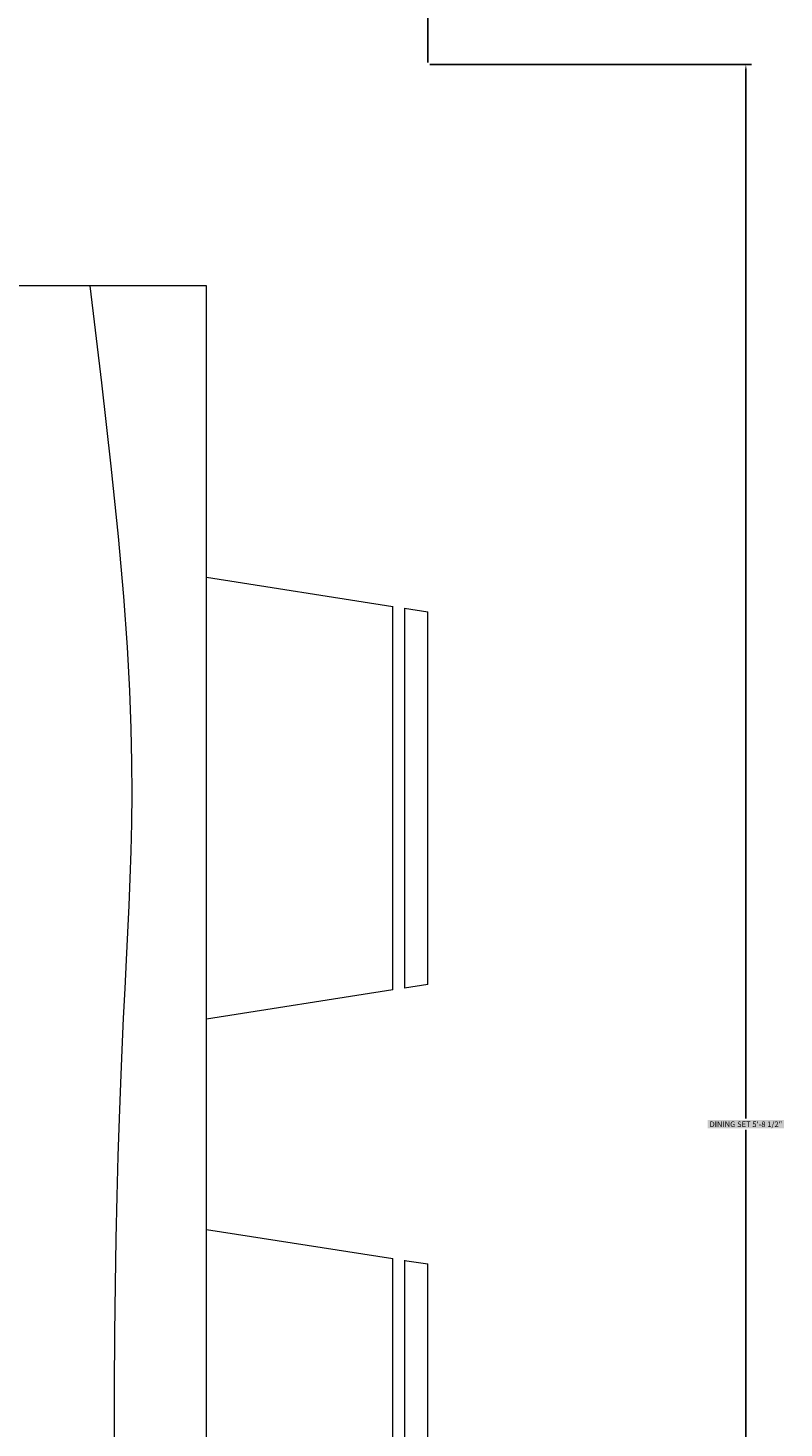
# Model space of a CAD drawing. Units: inches. Extents: x -301 to 715, y -607 to 364.
# Tile 112 of 141: x -12 to 12, y 147 to 192. Entities that reach past the tile are written whole.
import ezdxf

# ---------------------------------------------------------------- set-up
doc = ezdxf.new("R2010")
doc.units = ezdxf.units.IN
doc.header["$MEASUREMENT"] = 0
doc.layers.add('A-ANNO-DIMS', color=2, linetype='Continuous', lineweight=18)
doc.layers.add('A-FURN', color=8, linetype='Continuous', lineweight=18)
doc.styles.get("Standard").update_dxf_attribs({"font": 'arial.ttf'})
doc.dimstyles.get("Standard").update_dxf_attribs({"dimtxt": 0.18, "dimasz": 0.18, "dimexe": 0.18, "dimexo": 0.0625, "dimgap": 0.09, "dimtad": 0, "dimtih": 1, "dimtoh": 1, "dimdec": 1, "dimzin": 0, "dimdsep": 46, "dimlunit": 4, "dimtxsty": 'Standard', "dimcen": 0.09, "dimclrd": 3, "dimclre": 4, "dimclrt": 6, "dimadec": 0, "dimazin": 0, "dimtfac": 1, "dimtdec": 1, "dimtofl": 0, "dimtmove": 0, "dimatfit": 3, "dimfxl": 1, "dimtfill": 2, "dimtfillclr": 51, "dimtolj": 1, "dimtzin": 0, "dimarcsym": 0})

# ---------------------------------------------------------------- blocks, each defined once
blk = doc.blocks.new('Dining Set - 36 x 72 in.')
for p, q in [((36, -18), (36, 18)), ((-36, -18), (36, -18)), ((-4.5152, -17.99762), (-5.7655, -25.99928)), ((5.7657, -26.0006), (4.5153, -17.99762)), ((23.4848, -17.99762), (22.2345, -25.99928)), ((-22.2304, -26), (-5.7608, -26)), ((5.7696, -26), (22.2392, -26)), ((-5.8416, -26.5), (-22.1534, -26.5)), ((-5.8437, -26.49967), (-6, -27.5)), ((6, -27.5), (5.8438, -26.50044)), ((22.1584, -26.5), (5.8466, -26.5)), ((22.1563, -26.49967), (22, -27.5)), ((-22, -27.5), (-6, -27.5)), ((6, -27.5), (22, -27.5))]:
    blk.add_line(p, q)
blk.add_lwpolyline([(-13.97, -14.04671), (-11.3027, -14.04297), (-8.9724, -14.05681), (-6.875, -14.08334), (-4.9224, -14.11833), (-3.0905, -14.16016), (-1.3709, -14.20785), (0.2448, -14.26042), (1.7647, -14.3169), (3.1973, -14.3763), (4.5507, -14.43767), (5.8333, -14.5), (7.0554, -14.5621), (8.235, -14.62175), (9.3922, -14.67652), (10.5469, -14.72396), (11.7192, -14.76164), (12.929, -14.78711), (14.1965, -14.79794), (15.5417, -14.79167), (16.9933, -14.76424), (18.6152, -14.70508), (20.4804, -14.60197), (22.6615, -14.44271), (25.2312, -14.21509), (28.2624, -13.9069), (31.8277, -13.50594), (36, -13)])
blk = doc.blocks.new('*D128')
at = {"layer": 'A-ANNO-DIMS', "color": 4, "lineweight": -2, "transparency": 16777216}
for p, q in [((0.532, 191.307), (10.93, 191.307)), ((0.532, 122.765), (10.93, 122.765))]:
    blk.add_line(p, q, dxfattribs=at)
at = {"layer": 'A-ANNO-DIMS', "color": 3, "lineweight": -2, "transparency": 16777216}
for p, q in [((10.75, 191.127), (10.75, 157.219)), ((10.75, 122.945), (10.75, 156.853))]:
    blk.add_line(p, q, dxfattribs=at)
at = {"layer": 'A-ANNO-DIMS', "color": 3, "transparency": 16777216}
for points in [[(10.72, 191.127), (10.78, 191.127), (10.75, 191.307)], [(10.72, 122.945), (10.78, 122.945), (10.75, 122.765)]]:
    blk.add_solid(points, dxfattribs=at)
at = {"layer": 'Defpoints', "color": 0, "transparency": 16777216}
for p in [(0.469, 191.307), (10.75, 191.307), (0.469, 122.765)]:
    blk.add_point(p, dxfattribs=at)
at = {"layer": 'A-ANNO-DIMS', "color": 6, "transparency": 16777216, "insert": (10.75, 157.036), "char_height": 0.18, "attachment_point": 5, "bg_fill": 1, "box_fill_scale": 1.25, "bg_fill_color": 51, "bg_fill_transparency": 0}
blk.add_mtext('\\A1;DINING SET 5\'-8 1/2"', dxfattribs=at)
blk = doc.blocks.new('*D129')
at = {"layer": 'A-ANNO-DIMS', "color": 4, "lineweight": -2, "transparency": 16777216}
for p, q in [((-40.957, 191.37), (-40.957, 201.768)), ((0.469, 191.37), (0.469, 201.768))]:
    blk.add_line(p, q, dxfattribs=at)
at = {"layer": 'A-ANNO-DIMS', "color": 3, "lineweight": -2, "transparency": 16777216}
for p, q in [((-40.777, 201.588), (-20.783, 201.588)), ((0.289, 201.588), (-19.705, 201.588))]:
    blk.add_line(p, q, dxfattribs=at)
at = {"layer": 'A-ANNO-DIMS', "color": 3, "transparency": 16777216}
for points in [[(-40.777, 201.618), (-40.777, 201.558), (-40.957, 201.588)], [(0.289, 201.618), (0.289, 201.558), (0.469, 201.588)]]:
    blk.add_solid(points, dxfattribs=at)
at = {"layer": 'Defpoints', "color": 0, "transparency": 16777216}
for p in [(-40.957, 201.588), (-40.957, 191.307), (0.469, 191.307)]:
    blk.add_point(p, dxfattribs=at)
at = {"layer": 'A-ANNO-DIMS', "color": 6, "transparency": 16777216, "insert": (-20.244, 201.588), "char_height": 0.18, "attachment_point": 5, "bg_fill": 1, "box_fill_scale": 1.25, "bg_fill_color": 51, "bg_fill_transparency": 0}
blk.add_mtext('\\A1;3\'-5 1/2"', dxfattribs=at)

msp = doc.modelspace()

# ---------------------------------------------------------------- block references
at = {"layer": 'A-FURN', "xscale": 0.753207081168398, "yscale": 0.753207081168398, "zscale": 0.753207081168398, "rotation": 90}
msp.add_blockref('Dining Set - 36 x 72 in.', (-20.244, 157.036), dxfattribs=at)

# ---------------------------------------------------------------- dimensions: what is measured, and where the dimension line sits
at = {"layer": 'A-ANNO-DIMS'}
dim = msp.add_linear_dim(base=(-40.957, 201.588), p1=(0.469, 191.307), p2=(-40.957, 191.307), angle=180, dimstyle='Standard', override={"dimdec": 1, "dimlfac": 1, "dimrnd": 0, "dimzin": 1, "dimdsep": 46, "dimlunit": 4, "dimfrac": 2}, dxfattribs=at)
dim.commit()
dim.dimension.update_dxf_attribs({"geometry": '*D129', "text_midpoint": (-20.244, 201.588)})
dim = msp.add_linear_dim(base=(10.75, 191.307), p1=(0.469, 122.765), p2=(0.469, 191.307), angle=90, text='DINING SET <>', dimstyle='Standard', override={"dimdec": 1, "dimlfac": 1, "dimrnd": 0, "dimzin": 1, "dimdsep": 46, "dimlunit": 4, "dimfrac": 2}, dxfattribs=at)
dim.commit()
dim.dimension.update_dxf_attribs({"geometry": '*D128', "text_midpoint": (10.75, 157.036)})

doc.saveas('drawing.dxf')
